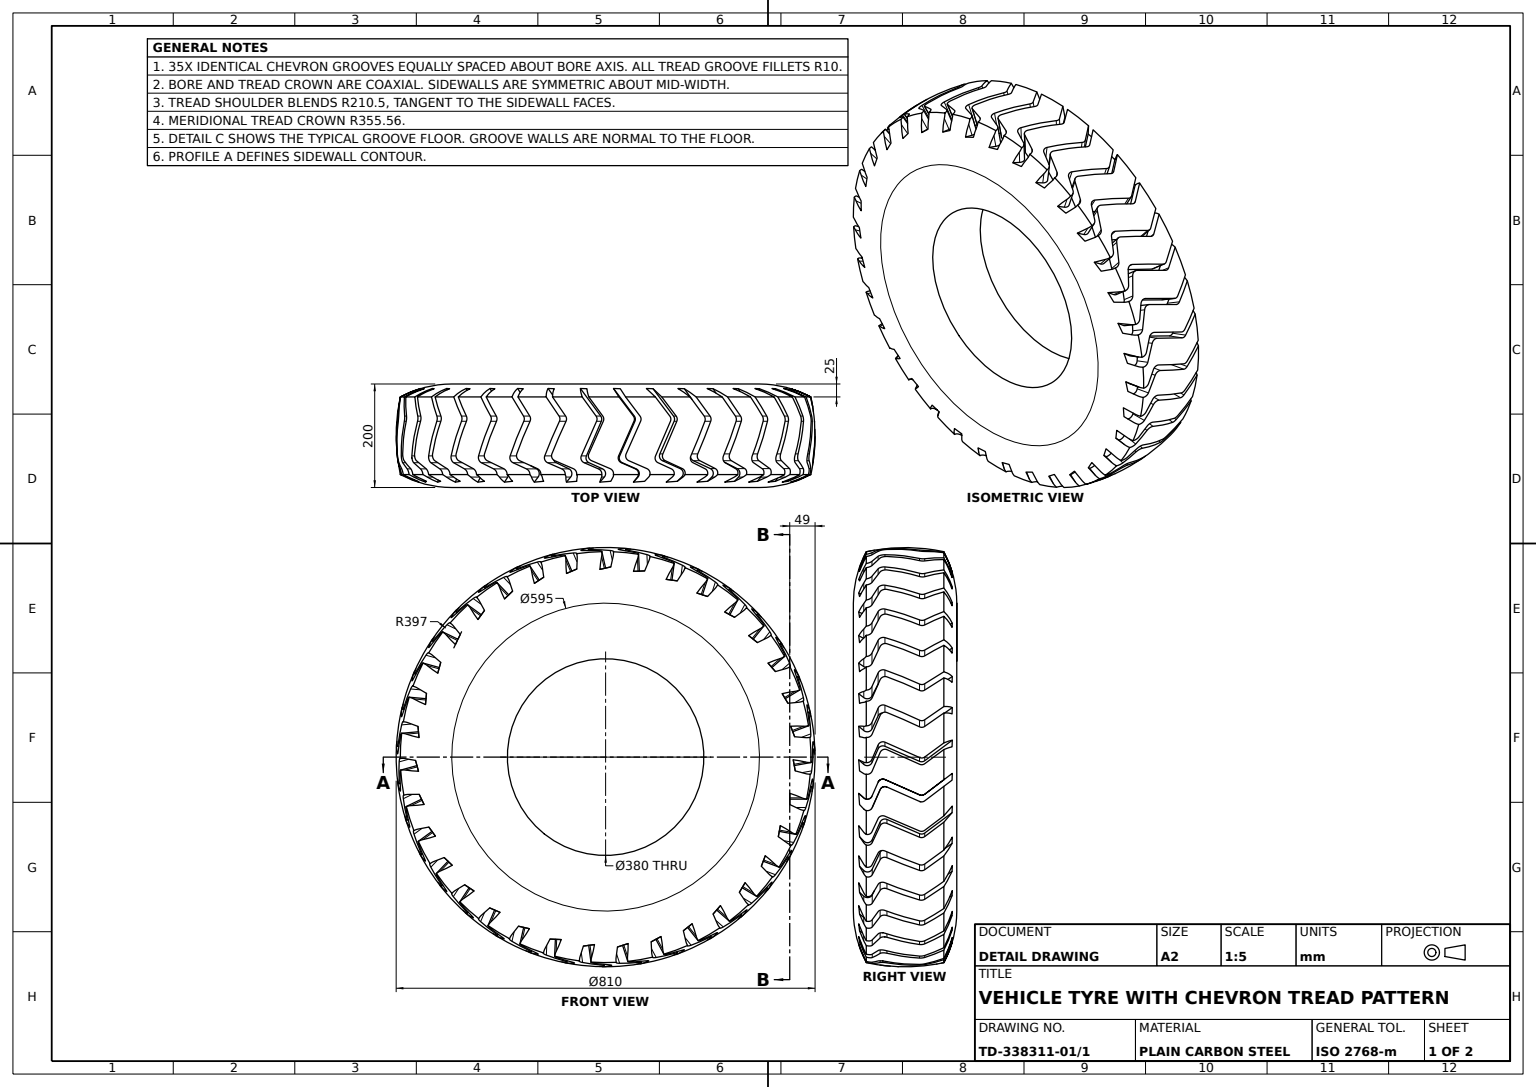
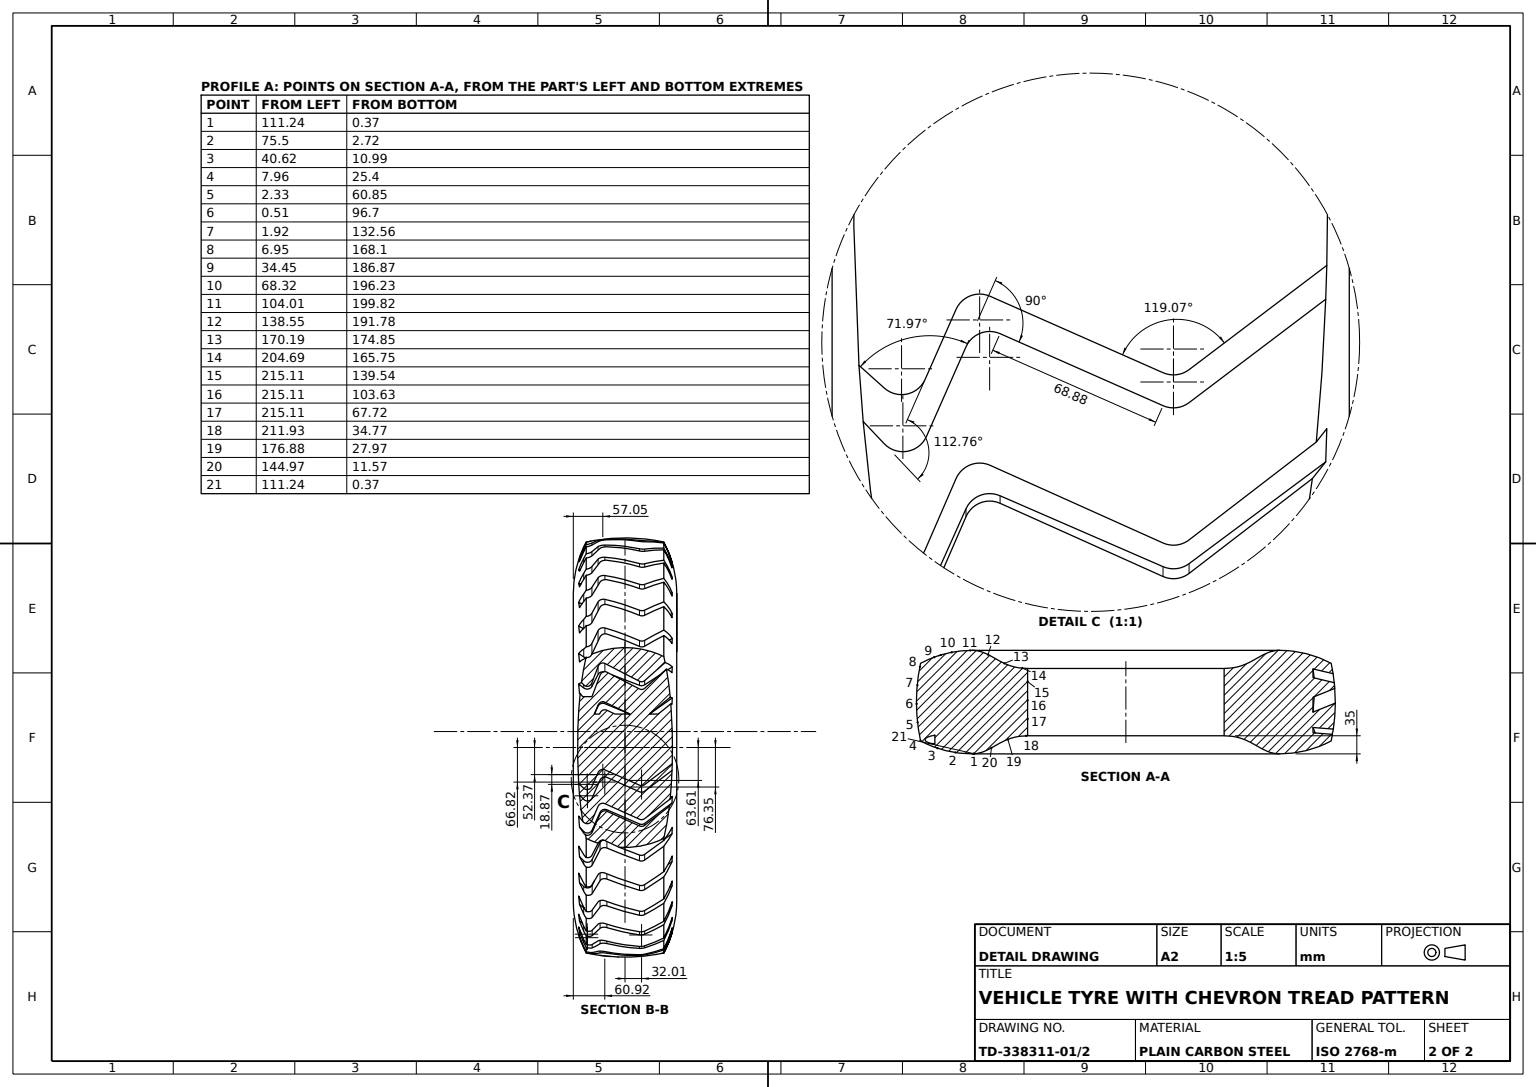
from build123d import *

# Parameters (mm, degrees)
TREAD_GROOVE_CUT_DEPTH         = 54
TREAD_GROOVE_PATTERN_35X_COUNT = 35


with BuildPart() as part:
    # Tyre Section Profile → Tyre Body (revolve)
    with BuildSketch(Plane.XY, mode=Mode.PRIVATE) as tyre_body_sk:
        with BuildLine():
            ThreePointArc((75, 397), (37.712729946, 402.994343246), (0, 405))
            ThreePointArc((0, 405), (-37.712729946, 402.994343246), (-75, 397))
            ThreePointArc((-75, 397), (-93.654355713, 348.796320531), (-100, 297.5))
            add(Edge.make_bspline(
                [(-100, 297.5), (-100, 259.166666667), (-65, 244.027106856), (-65, 190)],
                knots=[0, 0, 0, 0, 1, 1, 1, 1], degree=3))
            Line((-65, 190), (-45, 190))
            Line((-45, 190), (65, 190))
            add(Edge.make_bspline(
                [(100, 297.5), (100, 259.166666667), (65, 244.027106856), (65, 190)],
                knots=[0, 0, 0, 0, 1, 1, 1, 1], degree=3))
            ThreePointArc((100, 297.5), (93.654355713, 348.796320531), (75, 397))
        make_face()
    revolve(tyre_body_sk.sketch.rotate(Axis((0, 0, 0), (1, 0, 0)), 90), axis=Axis((0, 0, 0), (1, 0, 0)))

    # Tread Groove Sketch → Tread Groove Cut (cut)
    with BuildSketch(Plane(origin=(0, 410, 0), x_dir=(1, 0, 0), z_dir=(0, 1, 0))):
        with BuildLine():
            Line((-123.916969576, 19.384841315), (-38.043911448, 84.329802174))
            ThreePointArc((-38.043911448, 84.329802174), (-33.167325949, 86.286967979), (-27.971695415, 85.501469742))
            Line((-27.971695415, 85.501469742), (35.039444666, 57.67154954))
            ThreePointArc((35.039444666, 57.67154954), (42.691053069, 57.49397533), (48.227121186, 62.778915591))
            Line((48.227121186, 62.778915591), (63.484280853, 97.323428045))
            ThreePointArc((63.484280853, 97.323428045), (70.930840079, 103.137547419), (79.895596876, 100.156211485))
            Line((79.895596876, 100.156211485), (123.916969576, 53.631394305))
            Line((123.916969576, 53.631394305), (123.916969576, 39.182987719))
            Line((123.916969576, 39.182987719), (79.816539674, 78.689722367))
            ThreePointArc((79.816539674, 78.689722367), (71.038012661, 81.017093134), (63.996525847, 75.281532599))
            Line((63.996525847, 75.281532599), (52.093157093, 48.330509005))
            ThreePointArc((52.093157093, 48.330509005), (46.557088976, 43.045568744), (38.905480572, 43.223142954))
            Line((38.905480572, 43.223142954), (-27.971695415, 72.760562348))
            ThreePointArc((-27.971695415, 72.760562348), (-33.167325949, 73.546060585), (-38.043911448, 71.58889478))
            Line((-38.043911448, 71.58889478), (-123.916969576, 6.643933921))
            Line((-123.916969576, 6.643933921), (-123.916969576, 19.384841315))
        make_face()
    tread_groove_cut = extrude(amount=-TREAD_GROOVE_CUT_DEPTH, mode=Mode.SUBTRACT)

    # Tread Groove Pattern 35x: Tread Groove Cut ×35 about axis
    tread_groove_pattern_35x_axis = Axis((0, 0, 0), (1, 0, 0))
    for i in range(1, TREAD_GROOVE_PATTERN_35X_COUNT):
        add(tread_groove_cut.rotate(tread_groove_pattern_35x_axis, i * 360 / TREAD_GROOVE_PATTERN_35X_COUNT), mode=Mode.SUBTRACT)


solid = part.part
